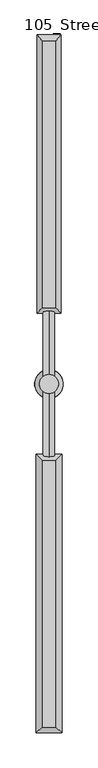
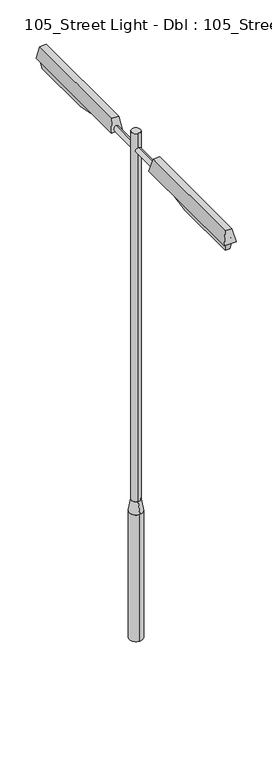
"""IFC4 building model written with IfcOpenShell, lengths in millimetres: light fixture geometry, 105_Street Light - Dbl : 105_Street Light - Dbl."""

from ifc_helpers import new_model, si_unit, point, frame, frame_2d, origin, origin_with_axes, place, context, project, spatial, polyline, circle_curve, trimmed, segment, composite_curve, outline, extrude, faceted_brep, source, transform, mapped, element, save
from ifc_brep_helpers import plane_surface, revolved_surface, advanced_brep


def light_fixture_105_street_light_dbl_105_street_light_dbl_4055396a(model_context):
    return source(origin(), model_context, "Body", "SolidModel", [
        extrude(outline(composite_curve([segment(trimmed(circle_curve(frame_2d((43.5647283, 0.0)), 50.0), [point((43.5647283, 50.0))], [point((43.5647283, -50.0))], False, "CARTESIAN"), True, "CONTINUOUS"), segment(trimmed(circle_curve(frame_2d((43.5647283, 0.0)), 50.0), [point((43.5647283, -50.0))], [point((43.5647283, 50.0))], False, "CARTESIAN"), True, "CONTINUOUS")], self_intersect=False)), frame((0.0, 0.0, 1640.0), z_axis=(0.0, 0.0, 1.0), x_axis=(1.0, 0.0, 0.0)), (0.0, 0.0, 1.0), 4360.0),
        advanced_brep(
        [(43.5647283, 50.0, 1640.0), (43.5647283, -50.0, 1640.0), (43.5647283, 75.0, 1500.0), (43.5647283, -75.0, 1500.0)],
        [
            (0, 1, circle_curve(frame((43.5647283, 0.0, 1640.0), z_axis=(0.0, 0.0, 1.0), x_axis=(0.0, 1.0, 0.0)), 50.0)),
            (1, 0, circle_curve(frame((43.5647283, 0.0, 1640.0), z_axis=(0.0, 0.0, 1.0), x_axis=(0.0, -1.0, 0.0)), 50.0)),
            (2, 3, circle_curve(frame((43.5647283, 0.0, 1500.0), z_axis=(0.0, 0.0, -1.0), x_axis=(0.0, -1.0, 0.0)), 75.0)),
            (3, 2, circle_curve(frame((43.5647283, 0.0, 1500.0), z_axis=(0.0, 0.0, -1.0), x_axis=(0.0, 1.0, 0.0)), 75.0)),
            (3, 1),
            (0, 2),
        ],
        [
            plane_surface(frame((43.5647283, 0.0, 1640.0), z_axis=(0.0, 0.0, 1.0), x_axis=(-1.0, 0.0, 0.0))),
            plane_surface(frame((43.5647283, 0.0, 1500.0), z_axis=(0.0, 0.0, -1.0), x_axis=(-1.0, 0.0, 0.0))),
            revolved_surface(polyline([(43.5647283, 50.0, 1640.0), (43.5647283, 75.0, 1500.0)]), (43.5647283, 0.0, 1920.0), (0.0, 0.0, -1.0)),
            revolved_surface(polyline([(43.5647283, -50.0, 1640.0), (43.5647283, -75.0, 1500.0)]), (43.5647283, 0.0, 1920.0), (0.0, 0.0, -1.0)),
        ],
        [
            (0, [[1, 2]]),
            (1, [[3, 4]]),
            (2, [[-4, 5, -1, 6]]),
            (3, [[-3, -6, -2, -5]]),
        ],
    ),
        extrude(outline(composite_curve([segment(trimmed(circle_curve(frame_2d((43.5647283, 0.0)), 75.0), [point((43.5647283, 75.0))], [point((43.5647283, -75.0))], False, "CARTESIAN"), True, "CONTINUOUS"), segment(trimmed(circle_curve(frame_2d((43.5647283, 0.0)), 75.0), [point((43.5647283, -75.0))], [point((43.5647283, 75.0))], False, "CARTESIAN"), True, "CONTINUOUS")], self_intersect=False)), origin_with_axes(), (0.0, 0.0, 1.0), 1500.0),
        extrude(outline(composite_curve([segment(trimmed(circle_curve(frame_2d((5800.0, 43.5647283)), 30.0), [point((5830.0, 43.5647283))], [point((5770.0, 43.5647283))], False, "CARTESIAN"), True, "CONTINUOUS"), segment(trimmed(circle_curve(frame_2d((5800.0, 43.5647283)), 30.0), [point((5770.0, 43.5647283))], [point((5830.0, 43.5647283))], False, "CARTESIAN"), True, "CONTINUOUS")], self_intersect=False)), frame((0.0, -1800.0, 0.0), z_axis=(0.0, 1.0, 0.0), x_axis=(0.0, 0.0, 1.0)), (0.0, 0.0, 1.0), 3600.0),
        faceted_brep([(81.0647283, -1800.0, 5919.2599613), (81.0647283, -400.0, 5919.2599613), (6.0647283, -400.0, 5919.2599613), (6.0647283, -1800.0, 5919.2599613), (111.0647283, -1830.0, 5770.0), (-23.9352717, -1830.0, 5770.0), (-23.9352717, -370.0, 5770.0), (111.0647283, -370.0, 5770.0)], [[[0, 1, 2, 3]], [[4, 5, 6, 7]], [[4, 7, 1, 0]], [[7, 6, 2, 1]], [[6, 5, 3, 2]], [[5, 4, 0, 3]]]),
        faceted_brep([(68.5647283, -1000.0, 5670.0), (68.5647283, -1775.0, 5670.0), (18.5647283, -1775.0, 5670.0), (18.5647283, -1000.0, 5670.0), (81.0647283, -620.0, 5770.0), (6.0647283, -620.0, 5770.0), (6.0647283, -1800.0, 5770.0), (81.0647283, -1800.0, 5770.0)], [[[0, 1, 2, 3]], [[4, 5, 6, 7]], [[4, 7, 1, 0]], [[7, 6, 2, 1]], [[6, 5, 3, 2]], [[5, 4, 0, 3]]]),
        faceted_brep([(6.0647283, 1800.0, 5919.2599613), (6.0647283, 400.0, 5919.2599613), (81.0647283, 400.0, 5919.2599613), (81.0647283, 1800.0, 5919.2599613), (-19.0941637, 1829.9920379, 5770.0), (106.2236203, 1829.9920379, 5770.0), (106.2236203, 369.9920379, 5770.0), (-19.0941637, 369.9920379, 5770.0)], [[[0, 1, 2, 3]], [[4, 5, 6, 7]], [[4, 7, 1, 0]], [[7, 6, 2, 1]], [[6, 5, 3, 2]], [[5, 4, 0, 3]]]),
        faceted_brep([(68.5647283, 1775.0, 5670.0), (68.5647283, 1025.0, 5670.0), (18.5647283, 1025.0, 5670.0), (18.5647283, 1775.0, 5670.0), (81.0647283, 1800.0, 5770.0), (6.0647283, 1800.0, 5770.0), (6.0647283, 620.0, 5770.0), (81.0647283, 620.0, 5770.0)], [[[0, 1, 2, 3]], [[4, 5, 6, 7]], [[4, 7, 1, 0]], [[7, 6, 2, 1]], [[6, 5, 3, 2]], [[5, 4, 0, 3]]]),
    ])


if __name__ == "__main__":
    model = new_model("IFC4")
    model_context = context("Model", 3, world=origin())
    ifc_project = project(units=[si_unit("LENGTHUNIT", "METRE", prefix="MILLI")], contexts=[model_context])
    site = spatial("IfcSite", under=ifc_project)
    building = spatial("IfcBuilding", under=site)
    placement = place(None, origin())
    light_fixture_105_street_light_dbl_105_street_light_dbl_shape = light_fixture_105_street_light_dbl_105_street_light_dbl_4055396a(model_context)
    element("IfcLightFixture", 1, ObjectType="105_Street Light - Dbl : 105_Street Light - Dbl", at=placement, inside=building, context=model_context, shape_type="MappedRepresentation", body=[
        mapped(light_fixture_105_street_light_dbl_105_street_light_dbl_shape, transform((0.0, 0.0, 0.0), x_axis=(1.0, 0.0, 0.0), y_axis=(0.0, 1.0, 0.0), z_axis=(0.0, 0.0, 1.0))),
    ])
    save(model, "model.ifc")

# Revit data of these elements
# Type "105_Street Light - Dbl : 105_Street Light - Dbl"
#   Keynote = "V"
#   Wattage = 500 W
#   built-in parameter 1150110 = 1 (stored number, unit not read)
#   built-in parameter 1114217 = 2.64 (stored number, unit not read)
#   built-in parameter 1150109 = 1 (stored number, unit not read)
#   built-in parameter 1150113 = 1 (stored number, unit not read)
#   built-in parameter 1150105 = 5910.3 (stored number, unit not read)
#   Lumens = 74271 lm
#   built-in parameter 1150115 = 1 (stored number, unit not read)
#   Light Source Symbol Size = 2' - 0"
#   built-in parameter 1150112 = 1 (stored number, unit not read)
#   built-in parameter 1150114 = 1 (stored number, unit not read)
#   built-in parameter 1150107 = 6000 (stored number, unit not read)
#   built-in parameter 1150106 = 59.103 (stored number, unit not read)
#   Height = 19' - 8.22047"
#   built-in parameter 1150104 = 13.8 (stored number, unit not read)
#   Base Height = 4' - 11.05512"
#   built-in parameter 1114218 = 1 (stored number, unit not read)
#   built-in parameter 1150133 = 10 (stored number, unit not read)
#   Arm Length = 5' - 10.86614"
#   built-in parameter 1150134 = 5
#   Color Filter = 16777215
#   Material Lamp Post = Paint - Black Matte
#   Material Lamp Glazing = Glass
#   Dimming Lamp Color Temperature Shift = (empty or 0)
#   Default Elevation = 0
# Element 1 (IfcLightFixture, "105_Street Light - Dbl : 105_Street Light - Dbl")
#   Materials on its faces: "Paint - Black Matte", "Glass"
# Materials
#   "Paint - Black Matte": colour RGB 0 0 0, transparency 0
#   "Glass": class "Glass", colour RGB 218 227 224, transparency 0.85, Description = "Soda Lime Glass", Cost = 0
